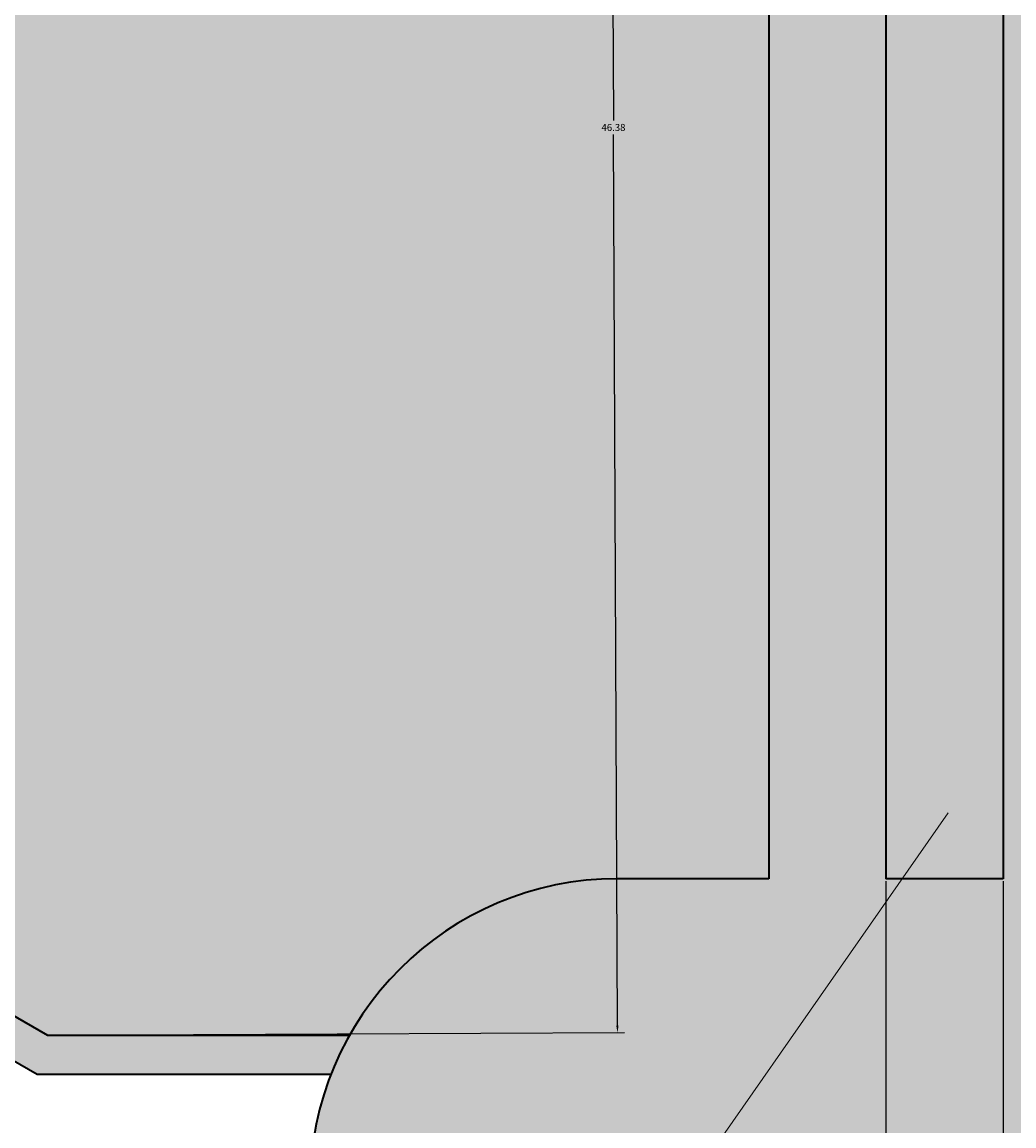
# Model space of a CAD drawing. Units: inches. Extents: x -1 to 292, y -3 to 199.
# Tile 8 of 52: x 43 to 68, y 45 to 73. Entities that reach past the tile are written whole.
import ezdxf

# ---------------------------------------------------------------- set-up
doc = ezdxf.new("R2010")
doc.units = ezdxf.units.IN
doc.header["$MEASUREMENT"] = 0
for name, color, linetype, lineweight in [('M-ANNO-LEAD', 2, 'Continuous', 18), ('M-DIMS', 2, 'Continuous', 18), ('M-EQPM', 7, 'Continuous', 35), ('M-PATT', 8, 'Continuous', 13)]:
    doc.layers.add(name, color=color, linetype=linetype, lineweight=lineweight)
doc.styles.get("Standard").update_dxf_attribs({"font": 'arial.ttf'})
doc.dimstyles.get("Standard").update_dxf_attribs({"dimtxt": 0.18, "dimasz": 0.18, "dimexe": 0.18, "dimexo": 0.0625, "dimgap": 0.09, "dimtad": 0, "dimtih": 1, "dimtoh": 1, "dimdec": 4, "dimzin": 0, "dimdsep": 46, "dimtxsty": 'Standard', "dimcen": 0.09, "dimadec": 0, "dimazin": 0, "dimtfac": 1, "dimtdec": 4, "dimtofl": 0, "dimtmove": 0, "dimatfit": 3, "dimfxl": 1, "dimtolj": 1, "dimtzin": 0, "dimarcsym": 0})

# ---------------------------------------------------------------- blocks, each defined once
blk = doc.blocks.new('BOILER-TUBE')
for p, q in [((0, 40.63), (0, 0)), ((3, 40.63), (3, 0))]:
    blk.add_line(p, q)
blk.add_lwpolyline([(3, 0), (0, 0)])
blk = doc.blocks.new('*D7')
at = {"layer": 'Defpoints', "color": 0, "transparency": 16777216}
for p in [(21.861, 54.582), (205.115, 54.582), (21.861, 39.982)]:
    blk.add_point(p, dxfattribs=at)
at = {"layer": 'M-DIMS', "color": 0, "lineweight": -2, "transparency": 16777216}
for p, q in [((21.861, 54.52), (21.861, 39.802)), ((205.115, 54.52), (205.115, 39.802)), ((22.041, 39.982), (113.033, 39.982)), ((204.935, 39.982), (113.944, 39.982))]:
    blk.add_line(p, q, dxfattribs=at)
at = {"layer": 'M-DIMS', "color": 0, "transparency": 16777216}
for points in [[(22.041, 40.012), (22.041, 39.952), (21.861, 39.982)], [(204.935, 40.012), (204.935, 39.952), (205.115, 39.982)]]:
    blk.add_solid(points, dxfattribs=at)
at = {"layer": 'M-DIMS', "color": 0, "transparency": 16777216, "insert": (113.488, 39.982), "char_height": 0.18, "attachment_point": 5}
blk.add_mtext('\\A1;183.25', dxfattribs=at)
blk = doc.blocks.new('*D8')
at = {"layer": 'Defpoints', "color": 0, "transparency": 16777216}
for p in [(-0.662, 126.765), (111.488, 126.765), (69.013, 25.514)]:
    blk.add_point(p, dxfattribs=at)
at = {"layer": 'M-DIMS', "color": 0, "lineweight": -2, "transparency": 16777216}
for p, q in [((111.426, 126.765), (-0.842, 126.765)), ((-0.662, 126.585), (-0.662, 76.321)), ((-0.662, 25.694), (-0.662, 75.958)), ((68.951, 25.514), (-0.842, 25.514))]:
    blk.add_line(p, q, dxfattribs=at)
at = {"layer": 'M-DIMS', "color": 0, "transparency": 16777216}
for points in [[(-0.692, 126.585), (-0.632, 126.585), (-0.662, 126.765)], [(-0.692, 25.694), (-0.632, 25.694), (-0.662, 25.514)]]:
    blk.add_solid(points, dxfattribs=at)
at = {"layer": 'M-DIMS', "color": 0, "transparency": 16777216, "insert": (-0.662, 76.14), "char_height": 0.18, "attachment_point": 5}
blk.add_mtext('\\A1;101.25', dxfattribs=at)
blk = doc.blocks.new('*D18')
at = {"layer": 'Defpoints', "color": 0, "transparency": 16777216}
for p in [(42.998, 93.64), (43.201, 47.261), (57.801, 47.325)]:
    blk.add_point(p, dxfattribs=at)
at = {"layer": 'M-DIMS', "color": 0, "lineweight": -2, "transparency": 16777216}
for p, q in [((43.06, 93.641), (57.778, 93.705)), ((57.598, 93.524), (57.698, 70.697)), ((57.8, 47.505), (57.7, 70.333)), ((43.264, 47.262), (57.981, 47.326))]:
    blk.add_line(p, q, dxfattribs=at)
at = {"layer": 'M-DIMS', "color": 0, "transparency": 16777216}
for points in [[(57.628, 93.525), (57.568, 93.524), (57.598, 93.704)], [(57.83, 47.506), (57.77, 47.505), (57.801, 47.325)]]:
    blk.add_solid(points, dxfattribs=at)
at = {"layer": 'M-DIMS', "color": 0, "transparency": 16777216, "insert": (57.699, 70.515), "char_height": 0.18, "attachment_point": 5}
blk.add_mtext('\\A1;46.38', dxfattribs=at)
blk = doc.blocks.new('*D19')
at = {"layer": 'Defpoints', "color": 0, "transparency": 16777216}
for p in [(64.679, 51.267), (67.679, 51.267), (67.679, -2.71)]:
    blk.add_point(p, dxfattribs=at)
at = {"layer": 'M-DIMS', "color": 0, "lineweight": -2, "transparency": 16777216}
for p, q in [((64.679, 51.205), (64.679, -2.89)), ((67.679, 51.205), (67.679, -2.89)), ((64.859, -2.71), (66.03, -2.71)), ((67.499, -2.71), (66.328, -2.71))]:
    blk.add_line(p, q, dxfattribs=at)
at = {"layer": 'M-DIMS', "color": 0, "transparency": 16777216}
for points in [[(64.859, -2.68), (64.859, -2.74), (64.679, -2.71)], [(67.499, -2.68), (67.499, -2.74), (67.679, -2.71)]]:
    blk.add_solid(points, dxfattribs=at)
at = {"layer": 'M-DIMS', "color": 0, "transparency": 16777216, "insert": (66.179, -2.71), "char_height": 0.18, "attachment_point": 5}
blk.add_mtext('\\A1;3', dxfattribs=at)
blk = doc.blocks.new('*D20')
at = {"layer": 'Defpoints', "color": 0, "transparency": 16777216}
for p in [(64.679, 51.267), (70.679, 51.267), (70.679, -2.71)]:
    blk.add_point(p, dxfattribs=at)
at = {"layer": 'M-DIMS', "color": 0, "lineweight": -2, "transparency": 16777216}
for p, q in [((64.679, 51.205), (64.679, -2.89)), ((70.679, 51.205), (70.679, -2.89)), ((64.859, -2.71), (67.529, -2.71)), ((70.499, -2.71), (67.828, -2.71))]:
    blk.add_line(p, q, dxfattribs=at)
at = {"layer": 'M-DIMS', "color": 0, "transparency": 16777216}
for points in [[(64.859, -2.68), (64.859, -2.74), (64.679, -2.71)], [(70.499, -2.68), (70.499, -2.74), (70.679, -2.71)]]:
    blk.add_solid(points, dxfattribs=at)
at = {"layer": 'M-DIMS', "color": 0, "transparency": 16777216, "insert": (67.679, -2.71), "char_height": 0.18, "attachment_point": 5}
blk.add_mtext('\\A1;6', dxfattribs=at)
blk = doc.blocks.new('*D23')
at = {"layer": 'Defpoints', "color": 0, "transparency": 16777216}
for p in [(21.861, 54.582), (64.679, 51.267), (64.679, -2.71)]:
    blk.add_point(p, dxfattribs=at)
at = {"layer": 'M-DIMS', "color": 0, "lineweight": -2, "transparency": 16777216}
for p, q in [((21.861, 54.52), (21.861, -2.89)), ((64.679, 51.205), (64.679, -2.89)), ((22.041, -2.71), (42.874, -2.71)), ((64.499, -2.71), (43.666, -2.71))]:
    blk.add_line(p, q, dxfattribs=at)
at = {"layer": 'M-DIMS', "color": 0, "transparency": 16777216}
for points in [[(22.041, -2.68), (22.041, -2.74), (21.861, -2.71)], [(64.499, -2.68), (64.499, -2.74), (64.679, -2.71)]]:
    blk.add_solid(points, dxfattribs=at)
at = {"layer": 'M-DIMS', "color": 0, "transparency": 16777216, "insert": (43.27, -2.71), "char_height": 0.18, "attachment_point": 5}
blk.add_mtext('\\A1;42.82', dxfattribs=at)

msp = doc.modelspace()

# ---------------------------------------------------------------- hatches: boundary and pattern name
at = {"layer": 'M-PATT'}
h = msp.add_hatch(color=256, dxfattribs=at)
h.set_gradient(color1=(237, 31, 36), color2=(242, 113, 114), tint=1, name='CYLINDER')
h.paths.add_polyline_path([(106.0735, 105.9941), (106.0735, 106.9941), (108.0603, 106.9941), (107.8488, 107.6501), (57.8007, 107.6501, 0.4142136), (49.9241, 99.7735), (52.3176, 101.3278), (55.0097, 99.7735), (57.4032, 101.3278), (60.0953, 99.7735), (62.4888, 101.3278), (65.1809, 99.7735), (67.5744, 101.3278), (70.2665, 99.7735), (72.66, 101.3278), (75.3521, 99.7735), (77.7456, 101.3278), (80.4377, 99.7735), (82.8312, 101.3278), (85.5233, 99.7735), (87.9168, 101.3278), (90.6089, 99.7735), (93.0024, 101.3278), (95.6945, 99.7735), (98.088, 101.3278), (100.7801, 99.7735), (103.1736, 101.3278), (105.8657, 99.7735), (108.2592, 101.3278), (110.9513, 99.7735), (113.3448, 101.3278), (116.0369, 99.7735), (118.4304, 101.3278), (121.1225, 99.7735), (123.516, 101.3278), (126.2082, 99.7735), (128.6016, 101.3278), (131.2938, 99.7735), (133.6872, 101.3278), (136.3794, 99.7735), (138.7728, 101.3278), (141.465, 99.7735), (143.8584, 101.3278), (146.5506, 99.7735), (148.944, 101.3278), (151.6362, 99.7735), (154.0296, 101.3278), (156.7218, 99.7735), (159.1152, 101.3278), (160.6222, 100.4578), (160.6222, 107.6501), (115.4883, 107.6501), (115.4883, 106.9941), (120.9032, 106.9941), (120.9032, 105.9941), (120.9032, 103.3981), (106.0735, 103.3981)])
h.paths.add_polyline_path([(169.176, 107.6501), (162.1623, 107.6501), (162.1623, 100.004), (164.2008, 101.3278), (166.893, 99.7735), (169.2864, 101.3278), (171.9786, 99.7735), (174.372, 101.3278), (177.0526, 99.7802, 0.4139642)])
h.paths.add_polyline_path([(111.4883, 107.6501), (107.8488, 107.6501), (108.0603, 106.9941), (111.4883, 106.9941)], flags=17)
h.paths.add_polyline_path([(61.6788, 91.897), (57.8007, 91.897, -0.1099266), (54.4604, 92.6403), (43.2011, 92.6403), (23.9502, 84.4688), (23.9502, 58.376), (43.2011, 47.2615), (50.9409, 47.2615, -0.2705926), (57.8007, 51.2672), (61.6788, 51.2672)])
h.paths.add_polyline_path([(73.6788, 91.897), (70.6788, 91.897), (70.6788, 51.2672), (73.6788, 51.2672)])
h.paths.add_polyline_path([(79.6788, 91.897), (76.6788, 91.897), (76.6788, 51.2672), (79.6788, 51.2672)])
h.paths.add_polyline_path([(67.6788, 91.897), (64.6788, 91.897), (64.6788, 51.2672), (67.6788, 51.2672)])
h.paths.add_polyline_path([(101.6788, 91.897), (82.6788, 91.897), (82.6788, 51.2672), (101.6788, 51.2672)])
h.paths.add_polyline_path([(107.6788, 91.897), (104.6788, 91.897), (104.6788, 51.2672), (107.6788, 51.2672)])
h.paths.add_polyline_path([(113.6788, 91.897), (110.6788, 91.897), (110.6788, 51.2672), (113.6788, 51.2672)])
h.paths.add_polyline_path([(119.6788, 91.897), (116.6788, 91.897), (116.6788, 51.2672), (119.6788, 51.2672)])
h.paths.add_polyline_path([(141.6788, 91.897), (122.6788, 91.897), (122.6788, 51.2672), (141.6788, 51.2672)])
h.paths.add_polyline_path([(147.6788, 91.897), (144.6788, 91.897), (144.6788, 51.2672), (147.6788, 51.2672)])
h.paths.add_polyline_path([(153.6788, 91.897), (150.6788, 91.897), (150.6788, 51.2672), (153.6788, 51.2672)])
h.paths.add_polyline_path([(159.6788, 91.897), (156.6788, 91.897), (156.6788, 51.2672), (159.6788, 51.2672)])
h.paths.add_polyline_path([(179.5897, 92.6403), (172.5163, 92.6403, -0.1099266), (169.176, 91.897), (162.6788, 91.897), (162.6788, 51.2672), (169.176, 51.2672, -0.2705926), (176.0358, 47.2615), (179.5897, 47.2615)])
h.paths.add_polyline_path([(203.0265, 84.4688), (183.7755, 92.6403), (181.5897, 92.6403), (181.5897, 47.2615), (183.7755, 47.2615), (203.0265, 58.376)])
h.paths.add_polyline_path([(184.4188, 61.52), (200.7224, 61.52), (200.7224, 77.7532), (184.4188, 77.7532)], flags=24)
h = msp.add_hatch(color=256, dxfattribs=at)
h.set_gradient(color1=(0, 255, 255), color2=(0, 255, 255), tint=1)
h.paths.add_polyline_path([(75.3521, 99.7735), (72.66, 101.3278), (70.2665, 99.7735), (67.5744, 101.3278), (65.1809, 99.7735), (62.4888, 101.3278), (60.0953, 99.7735), (57.4032, 101.3278), (55.0097, 99.7735), (52.3176, 101.3278), (49.9241, 99.7735, 0.4142136), (57.8007, 91.897), (61.6788, 91.897), (61.6788, 51.2672), (57.8007, 51.2672, 0.8088808), (54.5813, 36.2021), (65.0947, 51.2672), (64.6788, 51.2672), (64.6788, 91.897), (67.6788, 91.897), (67.6788, 51.2672), (65.0947, 51.2672), (54.5813, 36.2021, 0.1056561), (57.8007, 35.5141), (169.176, 35.5141, 1), (169.176, 51.2672), (162.6788, 51.2672), (162.6788, 91.897), (169.176, 91.897, 0.4144629), (177.0526, 99.7802), (174.372, 101.3278), (171.9786, 99.7735), (169.2864, 101.3278), (166.893, 99.7735), (164.2008, 101.3278), (162.1623, 100.004), (162.1623, 96.1027), (160.6222, 96.1027), (160.6222, 100.4578), (159.1152, 101.3278), (156.7218, 99.7735), (154.0296, 101.3278), (151.6362, 99.7735), (148.944, 101.3278), (146.5506, 99.7735), (143.8584, 101.3278), (141.465, 99.7735), (138.7728, 101.3278), (136.3794, 99.7735), (133.6872, 101.3278), (131.2938, 99.7735), (128.6016, 101.3278), (126.2082, 99.7735), (123.516, 101.3278), (121.1225, 99.7735), (118.4304, 101.3278), (116.0369, 99.7735), (113.3448, 101.3278), (110.9513, 99.7735), (108.2592, 101.3278), (105.8657, 99.7735), (103.1736, 101.3278), (100.7801, 99.7735), (98.088, 101.3278), (95.6945, 99.7735), (93.0024, 101.3278), (90.6089, 99.7735), (87.9168, 101.3278), (85.5233, 99.7735), (82.8312, 101.3278), (80.4377, 99.7735), (77.7456, 101.3278)])
h.paths.add_polyline_path([(79.6788, 91.897), (79.6788, 51.2672), (76.6788, 51.2672), (76.6788, 91.897)], flags=16)
h.paths.add_polyline_path([(73.6788, 91.897), (73.6788, 51.2672), (70.6788, 51.2672), (70.6788, 91.897)], flags=16)
h.paths.add_polyline_path([(82.6788, 91.897), (101.6788, 91.897), (101.6788, 51.2672), (82.6788, 51.2672)], flags=16)
h.paths.add_polyline_path([(104.6788, 91.897), (107.6788, 91.897), (107.6788, 51.2672), (104.6788, 51.2672)], flags=16)
h.paths.add_polyline_path([(110.6788, 91.897), (113.6788, 91.897), (113.6788, 51.2672), (110.6788, 51.2672)], flags=16)
h.paths.add_polyline_path([(116.6788, 91.897), (119.6788, 91.897), (119.6788, 51.2672), (116.6788, 51.2672)], flags=16)
h.paths.add_polyline_path([(122.6788, 91.897), (141.6788, 91.897), (141.6788, 51.2672), (144.6788, 51.2672), (144.6788, 91.897), (147.6788, 91.897), (147.6788, 51.2672), (122.6788, 51.2672)], flags=16)
h.paths.add_polyline_path([(150.6788, 91.897), (153.6788, 91.897), (153.6788, 51.2672), (150.6788, 51.2672)], flags=16)
h.paths.add_polyline_path([(156.6788, 91.897), (159.6788, 91.897), (159.6788, 51.2672), (156.6788, 51.2672)], flags=16)
h = msp.add_hatch(color=256, dxfattribs=at)
h.set_gradient(color1=(76, 38, 47), color2=(76, 38, 47), tint=1, name='CYLINDER')
h.paths.add_polyline_path([(40.8628, 91.6478), (40.3591, 92.5203), (23.9502, 85.5552), (23.9502, 84.4688)])
h.paths.add_polyline_path([(52.8586, 93.6403), (42.9977, 93.6403), (40.3591, 92.5203), (40.8628, 91.6478), (43.2011, 92.6403), (54.4604, 92.6403, -0.0601508)])
h.paths.add_polyline_path([(23.9502, 88.5821), (21.8612, 88.5821), (21.8612, 54.5821), (23.9502, 54.5821)])
h.paths.add_polyline_path([(23.9502, 58.376), (23.9502, 57.2213), (42.9332, 46.2615), (50.4659, 46.2615, -0.0351813), (50.9409, 47.2615), (43.2011, 47.2615)])
h.paths.add_polyline_path([(179.5897, 93.6403), (174.1181, 93.6403, -0.0601508), (172.5163, 92.6403), (179.5897, 92.6403)])
h.paths.add_polyline_path([(183.979, 93.6403), (181.5897, 93.6403), (181.5897, 92.6403), (183.7755, 92.6403), (203.0265, 84.4688), (203.0265, 85.5552)])
h.paths.add_polyline_path([(205.1155, 88.5821), (203.0265, 88.5821), (203.0265, 54.5821), (205.1155, 54.5821)])
h.paths.add_polyline_path([(203.0265, 57.2213), (203.0265, 58.376), (183.7755, 47.2615), (181.5897, 47.2615), (181.5897, 46.2615), (184.0435, 46.2615)])
h.paths.add_polyline_path([(179.5897, 47.2615), (176.0358, 47.2615, -0.0351813), (176.5107, 46.2615), (179.5897, 46.2615)])

# ---------------------------------------------------------------- linework, layer by layer
at = {"layer": 'M-ANNO-LEAD'}
msp.add_line((66.2726, 52.955), (49.017, 28.2287), dxfattribs=at)
at = {"layer": 'M-EQPM'}
msp.add_line((61.6788, 91.897), (61.6788, 51.2672), dxfattribs=at)
for points in [[(23.9502, 58.376), (43.2011, 47.2615), (50.9409, 47.2615)], [(23.9502, 57.2213), (42.9332, 46.2615), (50.4659, 46.2615)]]:
    msp.add_lwpolyline(points, dxfattribs=at)
msp.add_lwpolyline([(61.6788, 51.2672), (57.8007, 51.2672, 1), (57.8007, 35.5141), (169.176, 35.5141, 1), (169.176, 51.2672), (162.6788, 51.2672)], format="xyb", dxfattribs=at)

# ---------------------------------------------------------------- block references
msp.add_blockref('BOILER-TUBE', (64.679, 51.267), dxfattribs=at)

# ---------------------------------------------------------------- dimensions: what is measured, and where the dimension line sits
at = {"layer": 'M-DIMS'}
for base, p1, p2, angle, picture, middle in [((-0.6625, 126.765), (69.013, 25.5141), (111.4883, 126.765), 90, '*D8', (-0.6625, 76.1396)), ((57.801, 47.3255), (42.9977, 93.6403), (43.2011, 47.2615), 270.25134, '*D18', (57.6993, 70.5149)), ((21.8612, 39.9821), (205.1155, 54.5821), (21.8612, 54.5821), 180, '*D7', (113.4883, 39.9821))]:
    dim = msp.add_linear_dim(base=base, p1=p1, p2=p2, angle=angle, dimstyle='Standard', override={"dimdec": 2, "dimlfac": 1, "dimrnd": 0, "dimzin": 0, "dimdsep": 46, "dimlunit": 2}, dxfattribs=at)
    dim.commit()
    dim.dimension.update_dxf_attribs({"geometry": picture, "text_midpoint": middle})
for base, p1, p2, override, picture, middle in [((64.6788, -2.7104), (21.8612, 54.5821), (64.6788, 51.2672), {"dimdec": 2, "dimlfac": 1, "dimrnd": 0, "dimzin": 0, "dimdsep": 46, "dimlunit": 2}, '*D23', (43.27, -2.7104)), ((67.6788, -2.7104), (64.6788, 51.2672), (67.6788, 51.2672), {"dimdec": 0, "dimlfac": 1, "dimrnd": 0, "dimzin": 0, "dimdsep": 46, "dimlunit": 2}, '*D19', (66.1788, -2.7104)), ((70.6788, -2.7104), (64.6788, 51.2672), (70.6788, 51.2672), {"dimdec": 0, "dimlfac": 1, "dimrnd": 0, "dimzin": 0, "dimdsep": 46, "dimlunit": 2}, '*D20', (67.6788, -2.7104))]:
    dim = msp.add_linear_dim(base=base, p1=p1, p2=p2, dimstyle='Standard', override=override, dxfattribs=at)
    dim.commit()
    dim.dimension.update_dxf_attribs({"geometry": picture, "text_midpoint": middle})

doc.saveas('drawing.dxf')
